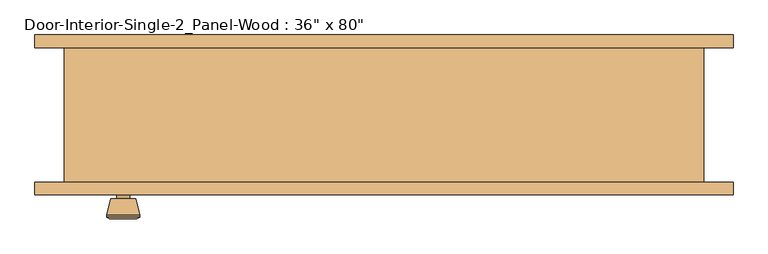
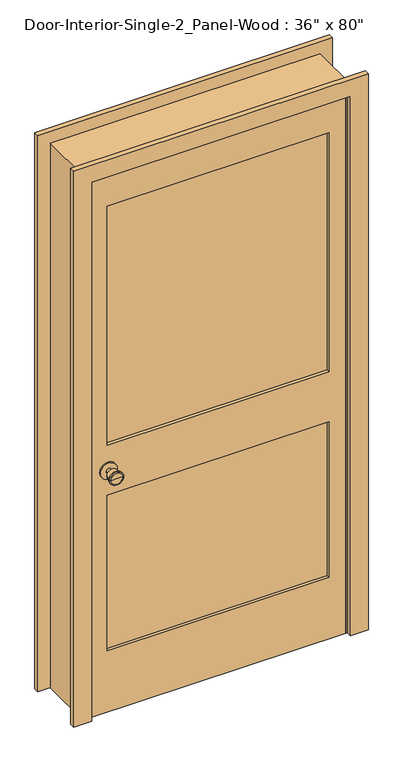
"""IFC4 building model written with IfcOpenShell, lengths in millimetres: door geometry."""

from ifc_helpers import new_model, si_unit, point, frame, frame_2d, origin, place, context, project, spatial, polyline, circle_curve, trimmed, segment, composite_curve, outline, extrude, faceted_brep, source, transform, mapped, element, save
from ifc_brep_helpers import plane_surface, cylinder_surface, revolved_surface, advanced_brep


def door_30de5629(model_context):
    return source(origin(), model_context, "Body", "SolidModel", [
        advanced_brep(
        [(-393.7, -57.5, 914.4), (-403.7, -57.5, 914.4), (-383.7, -57.5, 914.4), (-373.2241324, -8.5, 914.4), (-414.1758676, -8.5, 914.4), (-393.7, -8.5, 914.4), (-368.7, -10.3278681, 914.4), (-418.7, -10.3278681, 914.4), (-368.7, -13.7915463, 914.4), (-418.7, -13.7915463, 914.4), (-375.063764, -38.5, 914.4), (-412.336236, -38.5, 914.4), (-383.7, -38.5, 914.4), (-403.7, -38.5, 914.4)],
        [
            (0, 1),
            (1, 2, circle_curve(frame((-393.7, -57.5, 914.4), z_axis=(0.0, -1.0, 0.0), x_axis=(-1.0, 0.0, 0.0)), 10.0)),
            (2, 0),
            (2, 1, circle_curve(frame((-393.7, -57.5, 914.4), z_axis=(0.0, -1.0, 0.0), x_axis=(-1.0, 0.0, 0.0)), 10.0)),
            (3, 4, circle_curve(frame((-393.7, -8.5, 914.4), z_axis=(0.0, 1.0, 0.0), x_axis=(-1.0, 0.0, 0.0)), 20.4758676)),
            (4, 5),
            (5, 3),
            (4, 3, circle_curve(frame((-393.7, -8.5, 914.4), z_axis=(0.0, 1.0, 0.0), x_axis=(-1.0, 0.0, 0.0)), 20.4758676)),
            (6, 7, circle_curve(frame((-393.7, -10.3278681, 914.4), z_axis=(0.0, 1.0, 0.0), x_axis=(-1.0, 0.0, 0.0)), 25.0)),
            (7, 4),
            (3, 6),
            (7, 6, circle_curve(frame((-393.7, -10.3278681, 914.4), z_axis=(0.0, 1.0, 0.0), x_axis=(-1.0, 0.0, 0.0)), 25.0)),
            (8, 9, circle_curve(frame((-393.7, -13.7915463, 914.4), z_axis=(0.0, 1.0, 0.0), x_axis=(-1.0, 0.0, 0.0)), 25.0)),
            (9, 7),
            (6, 8),
            (9, 8, circle_curve(frame((-393.7, -13.7915463, 914.4), z_axis=(0.0, 1.0, 0.0), x_axis=(-1.0, 0.0, 0.0)), 25.0)),
            (10, 11, circle_curve(frame((-393.7, -38.5, 914.4), z_axis=(0.0, 1.0, 0.0), x_axis=(-1.0, 0.0, 0.0)), 18.636236)),
            (11, 9),
            (8, 10),
            (11, 10, circle_curve(frame((-393.7, -38.5, 914.4), z_axis=(0.0, 1.0, 0.0), x_axis=(-1.0, 0.0, 0.0)), 18.636236)),
            (12, 13, circle_curve(frame((-393.7, -38.5, 914.4), z_axis=(0.0, 1.0, 0.0), x_axis=(-1.0, 0.0, 0.0)), 10.0)),
            (13, 11),
            (10, 12),
            (13, 12, circle_curve(frame((-393.7, -38.5, 914.4), z_axis=(0.0, 1.0, 0.0), x_axis=(-1.0, 0.0, 0.0)), 10.0)),
            (1, 13),
            (12, 2),
        ],
        [
            plane_surface(frame((-393.7, -57.5, 914.4), z_axis=(0.0, -1.0, 0.0), x_axis=(-1.0, 0.0, 0.0))),
            plane_surface(frame((-393.7, -8.5, 914.4), z_axis=(0.0, 1.0, 0.0), x_axis=(-1.0, 0.0, 0.0))),
            revolved_surface(polyline([(-414.1758676, -8.5, 914.4), (-418.7, -10.3278681, 914.4)]), (-393.7, -57.5, 914.4), (0.0, -1.0, 0.0)),
            cylinder_surface(frame((-393.7, -57.5, 914.4), z_axis=(0.0, -1.0, 0.0), x_axis=(-1.0, 0.0, 0.0)), 25.0),
            revolved_surface(polyline([(-418.7, -13.7915463, 914.4), (-412.336236, -38.5, 914.4)]), (-393.7, -57.5, 914.4), (0.0, -1.0, 0.0)),
            plane_surface(frame((-393.7, -38.5, 914.4), z_axis=(0.0, -1.0, 0.0), x_axis=(-1.0, 0.0, 0.0))),
            cylinder_surface(frame((-393.7, -57.5, 914.4), z_axis=(0.0, -1.0, 0.0), x_axis=(-1.0, 0.0, 0.0)), 10.0),
        ],
        [
            (0, [[1, 2, 3]]),
            (0, [[-3, 4, -1]]),
            (1, [[5, 6, 7]]),
            (1, [[8, -7, -6]]),
            (2, [[9, 10, -5, 11]]),
            (2, [[12, -11, -8, -10]]),
            (3, [[13, 14, -9, 15]]),
            (3, [[16, -15, -12, -14]]),
            (4, [[17, 18, -13, 19]]),
            (4, [[20, -19, -16, -18]]),
            (5, [[21, 22, -17, 23]]),
            (5, [[24, -23, -20, -22]]),
            (6, [[-2, 25, -21, 26]]),
            (6, [[-4, -26, -24, -25]]),
        ],
    ),
        extrude(outline(composite_curve([segment(trimmed(circle_curve(frame_2d((914.4, -393.7)), 30.0), [point((914.4, -423.7))], [point((914.4, -363.7))], False, "CARTESIAN"), True, "CONTINUOUS"), segment(trimmed(circle_curve(frame_2d((914.4, -393.7)), 30.0), [point((914.4, -363.7))], [point((914.4, -423.7))], False, "CARTESIAN"), True, "CONTINUOUS")], self_intersect=False)), frame((0.0, -63.5, 0.0), z_axis=(0.0, 1.0, 0.0), x_axis=(0.0, 0.0, 1.0)), (0.0, 0.0, 1.0), 6.0),
        advanced_brep(
        [(-393.7, -104.425, 914.4), (-383.7, -104.425, 914.4), (-403.7, -104.425, 914.4), (-373.2241324, -153.425, 914.4), (-393.7, -153.425, 914.4), (-414.1758676, -153.425, 914.4), (-368.7, -151.5971319, 914.4), (-418.7, -151.5971319, 914.4), (-368.7, -148.1334537, 914.4), (-418.7, -148.1334537, 914.4), (-375.063764, -123.425, 914.4), (-412.336236, -123.425, 914.4), (-383.7, -123.425, 914.4), (-403.7, -123.425, 914.4)],
        [
            (0, 1),
            (1, 2, circle_curve(frame((-393.7, -104.425, 914.4), z_axis=(0.0, 1.0, 0.0), x_axis=(-1.0, 0.0, 0.0)), 10.0)),
            (2, 0),
            (2, 1, circle_curve(frame((-393.7, -104.425, 914.4), z_axis=(0.0, 1.0, 0.0), x_axis=(-1.0, 0.0, 0.0)), 10.0)),
            (3, 4),
            (4, 5),
            (5, 3, circle_curve(frame((-393.7, -153.425, 914.4), z_axis=(0.0, -1.0, 0.0), x_axis=(-1.0, 0.0, 0.0)), 20.4758676)),
            (3, 5, circle_curve(frame((-393.7, -153.425, 914.4), z_axis=(0.0, -1.0, 0.0), x_axis=(-1.0, 0.0, 0.0)), 20.4758676)),
            (6, 3),
            (5, 7),
            (7, 6, circle_curve(frame((-393.7, -151.5971319, 914.4), z_axis=(0.0, -1.0, 0.0), x_axis=(-1.0, 0.0, 0.0)), 25.0)),
            (6, 7, circle_curve(frame((-393.7, -151.5971319, 914.4), z_axis=(0.0, -1.0, 0.0), x_axis=(-1.0, 0.0, 0.0)), 25.0)),
            (8, 6),
            (7, 9),
            (9, 8, circle_curve(frame((-393.7, -148.1334537, 914.4), z_axis=(0.0, -1.0, 0.0), x_axis=(-1.0, 0.0, 0.0)), 25.0)),
            (8, 9, circle_curve(frame((-393.7, -148.1334537, 914.4), z_axis=(0.0, -1.0, 0.0), x_axis=(-1.0, 0.0, 0.0)), 25.0)),
            (10, 8),
            (9, 11),
            (11, 10, circle_curve(frame((-393.7, -123.425, 914.4), z_axis=(0.0, -1.0, 0.0), x_axis=(-1.0, 0.0, 0.0)), 18.636236)),
            (10, 11, circle_curve(frame((-393.7, -123.425, 914.4), z_axis=(0.0, -1.0, 0.0), x_axis=(-1.0, 0.0, 0.0)), 18.636236)),
            (12, 10),
            (11, 13),
            (13, 12, circle_curve(frame((-393.7, -123.425, 914.4), z_axis=(0.0, -1.0, 0.0), x_axis=(-1.0, 0.0, 0.0)), 10.0)),
            (12, 13, circle_curve(frame((-393.7, -123.425, 914.4), z_axis=(0.0, -1.0, 0.0), x_axis=(-1.0, 0.0, 0.0)), 10.0)),
            (1, 12),
            (13, 2),
        ],
        [
            plane_surface(frame((-393.7, -104.425, 914.4), z_axis=(0.0, 1.0, 0.0), x_axis=(-1.0, 0.0, 0.0))),
            plane_surface(frame((-393.7, -153.425, 914.4), z_axis=(0.0, -1.0, 0.0), x_axis=(-1.0, 0.0, 0.0))),
            revolved_surface(polyline([(-414.1758676, -153.425, 914.4), (-418.7, -151.5971319, 914.4)]), (-393.7, -104.425, 914.4), (0.0, 1.0, 0.0)),
            cylinder_surface(frame((-393.7, -104.425, 914.4), z_axis=(0.0, 1.0, 0.0), x_axis=(-1.0, 0.0, 0.0)), 25.0),
            revolved_surface(polyline([(-418.7, -148.1334537, 914.4), (-412.336236, -123.425, 914.4)]), (-393.7, -104.425, 914.4), (0.0, 1.0, 0.0)),
            plane_surface(frame((-393.7, -123.425, 914.4), z_axis=(0.0, 1.0, 0.0), x_axis=(-1.0, 0.0, 0.0))),
            cylinder_surface(frame((-393.7, -104.425, 914.4), z_axis=(0.0, 1.0, 0.0), x_axis=(-1.0, 0.0, 0.0)), 10.0),
        ],
        [
            (0, [[1, 2, 3]]),
            (0, [[-3, 4, -1]]),
            (1, [[5, 6, 7]]),
            (1, [[-6, -5, 8]]),
            (2, [[9, -7, 10, 11]]),
            (2, [[-10, -8, -9, 12]]),
            (3, [[13, -11, 14, 15]]),
            (3, [[-14, -12, -13, 16]]),
            (4, [[17, -15, 18, 19]]),
            (4, [[-18, -16, -17, 20]]),
            (5, [[21, -19, 22, 23]]),
            (5, [[-22, -20, -21, 24]]),
            (6, [[25, -23, 26, -2]]),
            (6, [[-26, -24, -25, -4]]),
        ],
    ),
        extrude(outline(composite_curve([segment(trimmed(circle_curve(frame_2d((914.4, -393.7)), 30.0), [point((914.4, -423.7))], [point((914.4, -363.7))], False, "CARTESIAN"), True, "CONTINUOUS"), segment(trimmed(circle_curve(frame_2d((914.4, -393.7)), 30.0), [point((914.4, -363.7))], [point((914.4, -423.7))], False, "CARTESIAN"), True, "CONTINUOUS")], self_intersect=False)), frame((0.0, -104.425, 0.0), z_axis=(0.0, 1.0, 0.0), x_axis=(0.0, 0.0, 1.0)), (0.0, 0.0, 1.0), 6.0),
        extrude(outline(polyline([(396.875, -75.1416667), (396.875, -86.7833333), (-396.875, -86.7833333), (-396.875, -75.1416667), (396.875, -75.1416667)])), frame((0.0, 0.0, 1009.65), z_axis=(0.0, 0.0, 1.0), x_axis=(1.0, 0.0, 0.0)), (0.0, 0.0, 1.0), 903.2875),
        extrude(outline(polyline([(396.875, -75.1416667), (396.875, -86.7833333), (-396.875, -86.7833333), (-396.875, -75.1416667), (396.875, -75.1416667)])), frame((0.0, 0.0, 231.775), z_axis=(0.0, 0.0, 1.0), x_axis=(1.0, 0.0, 0.0)), (0.0, 0.0, 1.0), 587.375),
        extrude(outline(polyline([(2032.0, -457.2), (0.0, -457.2), (0.0, 457.2), (2032.0, 457.2), (2032.0, -457.2)]), holes=[polyline([(1912.9375, -396.875), (1912.9375, 396.875), (1009.65, 396.875), (1009.65, -396.875), (1912.9375, -396.875)]), polyline([(819.15, -396.875), (819.15, 396.875), (231.775, 396.875), (231.775, -396.875), (819.15, -396.875)])]), frame((0.0, -98.425, 0.0), z_axis=(0.0, 1.0, 0.0), x_axis=(0.0, 0.0, 1.0)), (0.0, 0.0, 1.0), 34.925),
        faceted_brep([(482.6, -98.425, 0.0), (457.2, -98.425, 0.0), (457.2, -63.5, 0.0), (444.5, -63.5, 0.0), (444.5, -28.575, 0.0), (457.2, -28.575, 0.0), (457.2, 104.775, 0.0), (482.6, 104.775, 0.0), (482.6, 104.775, 2057.4), (482.6, -98.425, 2057.4), (457.2, 104.775, 2032.0), (-457.2, 104.775, 2032.0), (-457.2, 104.775, 0.0), (-482.6, 104.775, 0.0), (-482.6, 104.775, 2057.4), (457.2, -28.575, 2032.0), (444.5, -28.575, 2019.3), (-444.5, -28.575, 2019.3), (-444.5, -28.575, 0.0), (-457.2, -28.575, 0.0), (-457.2, -28.575, 2032.0), (444.5, -63.5, 2019.3), (457.2, -63.5, 2032.0), (-457.2, -63.5, 2032.0), (-457.2, -63.5, 0.0), (-444.5, -63.5, 0.0), (-444.5, -63.5, 2019.3), (457.2, -98.425, 2032.0), (-482.6, -98.425, 2057.4), (-482.6, -98.425, 0.0), (-457.2, -98.425, 0.0), (-457.2, -98.425, 2032.0)], [[[0, 1, 2, 3, 4, 5, 6, 7]], [[7, 8, 9, 0]], [[6, 10, 11, 12, 13, 14, 8, 7]], [[5, 15, 10, 6]], [[4, 16, 17, 18, 19, 20, 15, 5]], [[3, 21, 16, 4]], [[2, 22, 23, 24, 25, 26, 21, 3]], [[1, 27, 22, 2]], [[0, 9, 28, 29, 30, 31, 27, 1]], [[8, 14, 28, 9]], [[15, 20, 11, 10]], [[21, 26, 17, 16]], [[27, 31, 23, 22]], [[29, 13, 12, 19, 18, 25, 24, 30]], [[14, 13, 29, 28]], [[20, 19, 12, 11]], [[26, 25, 18, 17]], [[31, 30, 24, 23]]]),
        extrude(outline(polyline([(0.0, 527.05), (2101.85, 527.05), (2101.85, -527.05), (0.0, -527.05), (0.0, -463.55), (2038.35, -463.55), (2038.35, 463.55), (0.0, 463.55), (0.0, 527.05)])), frame((0.0, 104.775, 0.0), z_axis=(0.0, 1.0, 0.0), x_axis=(0.0, 0.0, 1.0)), (0.0, 0.0, 1.0), 19.05),
        extrude(outline(polyline([(0.0, 527.05), (2101.85, 527.05), (2101.85, -527.05), (0.0, -527.05), (0.0, -463.55), (2038.35, -463.55), (2038.35, 463.55), (0.0, 463.55), (0.0, 527.05)])), frame((0.0, -117.475, 0.0), z_axis=(0.0, 1.0, 0.0), x_axis=(0.0, 0.0, 1.0)), (0.0, 0.0, 1.0), 19.05),
    ])


if __name__ == "__main__":
    model = new_model("IFC4")
    model_context = context("Model", 3, world=origin())
    ifc_project = project(units=[si_unit("LENGTHUNIT", "METRE", prefix="MILLI")], contexts=[model_context])
    site = spatial("IfcSite", under=ifc_project)
    building = spatial("IfcBuilding", under=site)
    placement = place(None, origin())
    door_shape = door_30de5629(model_context)
    element("IfcDoor", 1, ObjectType="Door-Interior-Single-2_Panel-Wood : 36\" x 80\"", at=placement, inside=building, context=model_context, shape_type="MappedRepresentation", body=[
        mapped(door_shape, transform((0.0, 0.0, 0.0), x_axis=(1.0, 0.0, 0.0), y_axis=(0.0, 1.0, 0.0), z_axis=(0.0, 0.0, 1.0))),
    ])
    save(model, "model.ifc")

# Revit data of these elements
# Type "Door-Interior-Single-2_Panel-Wood : 36\" x 80\""
#   Type Mark = "10"
#   Assembly Code = "C1020300"
#   Analytic Construction = "Wooden"
#   Top Rail = 0' - 4 11/16"
#   Thickness = 0' - 1 3/8"
#   Thermal Resistance (R) = 2.5876 (h·ft²·°F)/BTU
#   Swing Angle [instance default] = 90.00°
#   Stiles = 0' - 2 3/8"
#   Rough Width = 3' - 2"
#   Rough Height = 6' - 9"
#   Lock Rail = 0' - 7 1/2"
#   Height = 6' - 8"
#   Width = 3' - 0"
#   Heat Transfer Coefficient (U) = 0.3865 BTU/(h·ft²·°F)
#   Bottom Rail = 0' - 9 1/8"
#   Trim Material = Cherry
#   Panel Material = Cherry
#   Frame Material = Cherry
#   Door Handle Material = Aluminum
#   Visual Light Transmittance = 0
#   Solar Heat Gain Coefficient = 0
#   Wall Closure = (empty or 0)
#   Function = (empty or 0)
# Element 1 (IfcDoor, "Door-Interior-Single-2_Panel-Wood : 36\" x 80\"")
#   Materials on its faces: "Cherry", "Aluminum"
# Materials
#   "Cherry": class "Wood", colour RGB 226 177 128, transparency 0, Description = "Prunus Serotina", Cost = 0
#   "Aluminum": class "Metal", colour RGB 247 247 247, transparency 0, Description = "Aluminum 6061", Cost = 0
